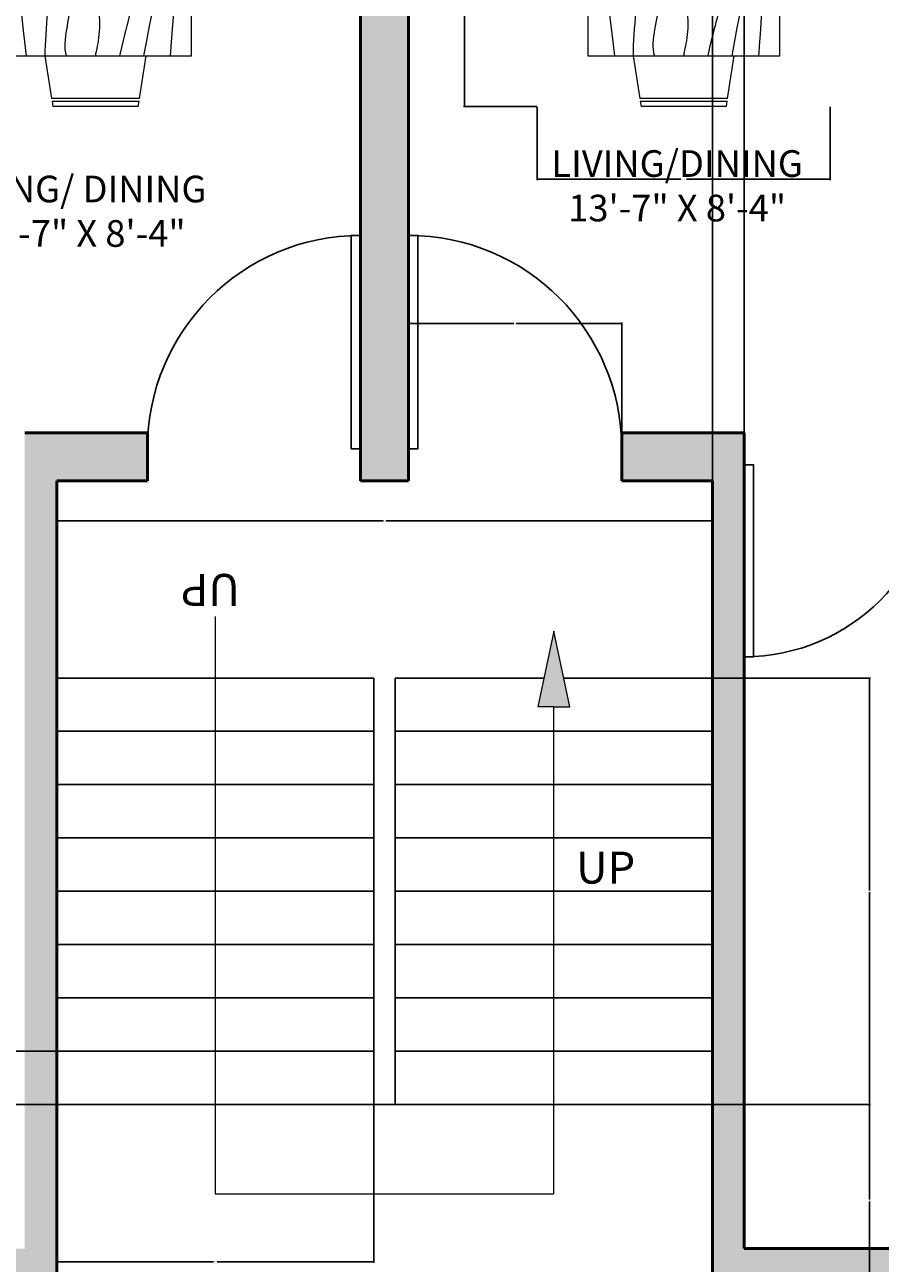
# Model space of a CAD drawing. Units: inches. Extents: x 2710 to 3197, y 524 to 1147.
# Tile 3 of 6: x 2885 to 3046, y 640 to 873. Entities that reach past the tile are written whole.
import ezdxf

# ---------------------------------------------------------------- set-up
doc = ezdxf.new("R2010")
doc.units = ezdxf.units.IN
for name, color, linetype, lineweight in [('A-ANNO-DIMS', 2, 'Continuous', 18), ('A-ANNO-SYMB', 1, 'Continuous', 18), ('A-ANNO-TEXT', 7, 'Continuous', 18), ('A-AREA-IDEN', 7, 'Continuous', 25), ('A-DOOR', 3, 'Continuous', 25), ('A-FLOR-STRS', 7, 'Continuous', 25), ('A-FURN', 8, 'Continuous', 18), ('A-WALL', 7, 'Continuous', 50), ('A-WALL-PATT', 74, 'Continuous', 13)]:
    doc.layers.add(name, color=color, linetype=linetype, lineweight=lineweight)
doc.styles.get("Standard").update_dxf_attribs({"font": 'arial.ttf'})
doc.dimstyles.get("Standard").update_dxf_attribs({"dimtxt": 0.18, "dimasz": 0.18, "dimexe": 0.18, "dimexo": 0.0625, "dimgap": 0.09, "dimtad": 0, "dimtih": 1, "dimtoh": 1, "dimdec": 4, "dimzin": 0, "dimdsep": 46, "dimtxsty": 'Standard', "dimcen": 0.09, "dimadec": 0, "dimazin": 0, "dimtfac": 1, "dimtdec": 4, "dimtofl": 0, "dimtmove": 0, "dimatfit": 3, "dimfxl": 1, "dimtolj": 1, "dimtzin": 0, "dimarcsym": 0})

# ---------------------------------------------------------------- blocks, each defined once
blk = doc.blocks.new('*U3')
for p, q in [((0, 0), (0, -6)), ((40, 0), (40, -6))]:
    blk.add_line(p, q)
blk.add_lwpolyline([(0, 0), (0, 40), (1.75, 40), (1.75, 0)], close=True)
blk.add_arc((0, 0), 40, 0, 90)
blk = doc.blocks.new('*U7')
for p, q in [((0, 0), (0, -6)), ((-40, 0), (-40, -6))]:
    blk.add_line(p, q)
blk.add_lwpolyline([(0, 0), (0, 40), (-1.75, 40), (-1.75, 0)], close=True)
blk.add_arc((0, 0), 40, 90, 180)
blk = doc.blocks.new('*U8')
for p, q in [((0, 0), (0, 6)), ((36, 0), (36, 6))]:
    blk.add_line(p, q)
blk.add_lwpolyline([(0, 0), (0, -36), (1.75, -36), (1.75, 0)], close=True)
blk.add_arc((0, 0), 36, 270, 0)
blk = doc.blocks.new('Dining Set - 36 x 72 in.')
for p, q in [((-22.2343, 26.00059), (-23.4847, 17.99762)), ((-22.2304, 26), (-5.7608, 26)), ((-22, 27.5), (-22.1562, 26.50042)), ((-5.8416, 26.5), (-22.1534, 26.5)), ((-22, 27.5), (-6, 27.5)), ((-5.8437, 26.49966), (-6, 27.5)), ((-4.5152, 17.99762), (-5.7655, 25.99926)), ((5.7657, 26.00059), (4.5153, 17.99762)), ((5.7696, 26), (22.2392, 26)), ((6, 27.5), (5.8438, 26.50042)), ((22.1584, 26.5), (5.8466, 26.5)), ((6, 27.5), (22, 27.5)), ((22.1563, 26.49966), (22, 27.5)), ((23.4848, 17.99762), (22.2345, 25.99926)), ((36, 18), (-36, 18)), ((-36, 18), (-36, -18)), ((36, -18), (36, 18)), ((-44.0006, 8.23428), (-35.9976, 9.48474)), ((44.0006, 8.23428), (35.9976, 9.48474)), ((-45.5, 8), (-44.5004, 8.15617)), ((-45.5, 8), (-45.5, -8)), ((-44.5, -8.15843), (-44.5, 8.15338)), ((-44, 8.23041), (-44, -8.23915)), ((44, 8.23041), (44, -8.23915)), ((44.5, -8.15843), (44.5, 8.15338)), ((45.5, 8), (44.5005, 8.15617)), ((45.5, 8), (45.5, -8)), ((-44.4997, -8.15631), (-45.5, -8)), ((-35.9976, -9.48476), (-43.9993, -8.2345)), ((35.9976, -9.48476), (43.9993, -8.2345)), ((44.4997, -8.15631), (45.5, -8)), ((-36, -18), (36, -18)), ((-22.2343, -26.0006), (-23.4847, -17.99762)), ((-4.5152, -17.99762), (-5.7655, -25.99928)), ((5.7657, -26.0006), (4.5153, -17.99762)), ((23.4848, -17.99762), (22.2345, -25.99928)), ((-22.2304, -26), (-5.7608, -26)), ((-22, -27.5), (-22.1562, -26.50044)), ((-5.8416, -26.5), (-22.1534, -26.5)), ((-22, -27.5), (-6, -27.5)), ((-5.8437, -26.49967), (-6, -27.5)), ((5.7696, -26), (22.2392, -26)), ((6, -27.5), (5.8438, -26.50044)), ((22.1584, -26.5), (5.8466, -26.5)), ((6, -27.5), (22, -27.5)), ((22.1563, -26.49967), (22, -27.5))]:
    blk.add_line(p, q)
for points in [[(-36, 15), (-31.1772, 14.97754), (-26.8079, 14.91406), (-22.8538, 14.81543), (-19.276, 14.6875), (-16.0362, 14.53613), (-13.0957, 14.36718), (-10.4159, 14.18652), (-7.9583, 14), (-5.6904, 13.81315), (-3.6035, 13.63021), (-1.6954, 13.45508), (0.0365, 13.29166), (1.5945, 13.14388), (2.9811, 13.01562), (4.1988, 12.9108), (5.25, 12.83333), (6.1393, 12.78613), (6.8802, 12.76823), (7.4883, 12.77767), (7.9792, 12.8125), (8.3685, 12.87077), (8.6719, 12.95052), (8.9049, 13.0498), (9.0833, 13.16666), (9.2205, 13.29899), (9.3216, 13.44401), (9.3895, 13.59879), (9.4271, 13.76041), (9.4373, 13.92594), (9.4232, 14.09245), (9.3875, 14.257), (9.3333, 14.41666), (9.2638, 14.56917), (9.1836, 14.71484), (9.0975, 14.85465), (9.0104, 14.98958), (8.9272, 15.1206), (8.8529, 15.2487), (8.7922, 15.37483), (8.75, 15.5), (8.7305, 15.62467), (8.7344, 15.74739), (8.7617, 15.86621), (8.8125, 15.97916), (8.8867, 16.08431), (8.9844, 16.17968), (9.1055, 16.26334), (9.25, 16.33333), (9.4189, 16.38802), (9.6172, 16.42708), (9.8506, 16.45052), (10.125, 16.45833), (10.4463, 16.45052), (10.8203, 16.42708), (11.2529, 16.38802), (11.75, 16.33333), (12.3184, 16.26318), (12.9694, 16.17838), (13.7151, 16.07991), (14.5677, 15.96875), (15.5395, 15.84586), (16.6426, 15.71224), (17.8893, 15.56884), (19.2917, 15.41666), (20.859, 15.25667), (22.5879, 15.08984), (24.4721, 14.91715), (26.5052, 14.73958), (28.6809, 14.5581), (30.9929, 14.3737), (33.4347, 14.18733), (36, 14)], [(-36, 10), (-28.9766, 10.14274), (-23.1725, 10.20442), (-18.4241, 10.19775), (-14.5677, 10.13541), (-11.4399, 10.03011), (-8.877, 9.89453), (-6.7154, 9.74137), (-4.7917, 9.58333), (-2.9698, 9.43082), (-1.2246, 9.28515), (0.4415, 9.14534), (2.026, 9.01041), (3.5266, 8.87939), (4.9408, 8.7513), (6.266, 8.62516), (7.5, 8.5), (8.6411, 8.37549), (9.6914, 8.2539), (10.6538, 8.13818), (11.5312, 8.03125), (12.3267, 7.93603), (13.043, 7.85547), (13.6831, 7.79248), (14.25, 7.75), (14.7471, 7.7303), (15.1797, 7.73307), (15.5537, 7.75732), (15.875, 7.80208), (16.1494, 7.86637), (16.3828, 7.94922), (16.5811, 8.04964), (16.75, 8.16666), (16.8944, 8.29915), (17.0143, 8.44531), (17.1089, 8.60319), (17.1771, 8.77083), (17.218, 8.94629), (17.2305, 9.1276), (17.2137, 9.31282), (17.1667, 9.5), (17.0895, 9.6875), (16.987, 9.875), (16.8649, 10.0625), (16.7292, 10.25), (16.5856, 10.4375), (16.4401, 10.625), (16.2985, 10.8125), (16.1667, 11), (16.05, 11.18733), (15.9518, 11.3737), (15.8752, 11.5581), (15.8229, 11.73958), (15.798, 11.91715), (15.8034, 12.08984), (15.842, 12.25667), (15.9167, 12.41666), (16.0295, 12.56836), (16.1784, 12.70833), (16.3605, 12.83268), (16.5729, 12.9375), (16.8127, 13.01888), (17.0768, 13.07291), (17.3625, 13.0957), (17.6667, 13.08333), (17.9894, 13.03312), (18.3418, 12.94726), (18.7382, 12.82918), (19.1927, 12.68229), (19.7195, 12.51001), (20.3327, 12.31575), (21.0465, 12.10294), (21.875, 11.875), (22.8357, 11.63354), (23.959, 11.37304), (25.2786, 11.08618), (26.8282, 10.76562), (28.6414, 10.40405), (30.752, 9.99414), (33.1936, 9.52856), (36, 9)], [(-36, 5.5), (-30.7157, 5.3348), (-26.069, 5.20963), (-21.9946, 5.11767), (-18.4271, 5.05208), (-15.3009, 5.00602), (-12.5508, 4.97265), (-10.1112, 4.94515), (-7.9167, 4.91666), (-5.909, 4.88167), (-4.0586, 4.83984), (-2.3429, 4.79215), (-0.7396, 4.73958), (0.7739, 4.6831), (2.22, 4.6237), (3.6213, 4.56233), (5, 4.5), (6.373, 4.43782), (7.7344, 4.3776), (9.0723, 4.32129), (10.375, 4.27083), (11.6309, 4.22819), (12.8281, 4.19531), (13.9551, 4.17415), (15, 4.16666), (15.954, 4.17448), (16.819, 4.19791), (17.6001, 4.23698), (18.3021, 4.29166), (18.9299, 4.36198), (19.4883, 4.44791), (19.9823, 4.54948), (20.4167, 4.66666), (20.7969, 4.79899), (21.1302, 4.94401), (21.4245, 5.09879), (21.6875, 5.26041), (21.9271, 5.42594), (22.1511, 5.59245), (22.3672, 5.757), (22.5834, 5.91666), (22.8065, 6.06868), (23.0404, 6.21093), (23.2879, 6.34147), (23.5521, 6.45833), (23.8358, 6.55957), (24.142, 6.64323), (24.4735, 6.70735), (24.8334, 6.75), (25.2235, 6.76969), (25.642, 6.76692), (26.0858, 6.74267), (26.5521, 6.69791), (27.0379, 6.63362), (27.5404, 6.55078), (28.0565, 6.45036), (28.5834, 6.33333), (29.1242, 6.19987), (29.7071, 6.04687), (30.3661, 5.87044), (31.1354, 5.66666), (32.0493, 5.43164), (33.142, 5.16146), (34.4475, 4.85221), (36, 4.5)], [(-36, -1), (-30.7915, -0.6591), (-26.0195, -0.38216), (-21.6519, -0.16284), (-17.6563, 0.00521), (-14.0005, 0.12833), (-10.6523, 0.21289), (-7.5796, 0.26522), (-4.75, 0.29166), (-2.134, 0.29793), (0.2878, 0.28711), (2.5317, 0.26163), (4.6146, 0.22396), (6.5529, 0.17651), (8.3633, 0.12174), (10.0623, 0.06209), (11.6667, 0), (13.1899, -0.06201), (14.6341, -0.1211), (15.9982, -0.17432), (17.2813, -0.21875), (18.4823, -0.25147), (19.6003, -0.26953), (20.6343, -0.27002), (21.5834, -0.25), (22.4481, -0.20768), (23.2357, -0.14584), (23.9549, -0.06836), (24.6146, 0.02083), (25.2235, 0.11784), (25.7904, 0.21875), (26.3241, 0.31966), (26.8334, 0.41666), (27.3265, 0.50618), (27.8099, 0.58593), (28.2894, 0.65397), (28.7709, 0.70833), (29.2601, 0.74707), (29.763, 0.76823), (30.2855, 0.76985), (30.8334, 0.75), (31.4088, 0.70784), (31.9994, 0.64713), (32.589, 0.57275), (33.1615, 0.48958), (33.7008, 0.4025), (34.1908, 0.3164), (34.6153, 0.23616), (34.9584, 0.16666), (35.2099, 0.11165), (35.3848, 0.07031), (35.504, 0.04069), (35.5886, 0.02083), (35.6594, 0.00879), (35.7377, 0.0026), (35.8442, 0.00032), (36, 0)], [(-36, -6.5), (-27.1843, -6.31267), (-20.084, -6.1263), (-14.469, -5.9419), (-10.1094, -5.76042), (-6.7752, -5.58285), (-4.2363, -5.41016), (-2.2629, -5.24333), (-0.625, -5.08334), (0.8708, -4.93099), (2.2715, -4.78646), (3.5872, -4.64974), (4.8281, -4.52084), (6.0046, -4.39974), (7.127, -4.28646), (8.2053, -4.18099), (9.25, -4.08334), (10.2705, -3.99382), (11.2734, -3.91407), (12.2647, -3.84603), (13.25, -3.79167), (14.2354, -3.75293), (15.2266, -3.73177), (16.2295, -3.73015), (17.25, -3.75), (18.2912, -3.79248), (19.3451, -3.85547), (20.4009, -3.93604), (21.4479, -4.03125), (22.4754, -4.13819), (23.4727, -4.25391), (24.4289, -4.37549), (25.3334, -4.5), (26.1785, -4.62492), (26.9694, -4.74935), (27.7145, -4.87281), (28.4219, -4.99479), (29.1, -5.11483), (29.7572, -5.23242), (30.4016, -5.34709), (31.0417, -5.45834), (31.6837, -5.56437), (32.3262, -5.65821), (32.9658, -5.73153), (33.599, -5.77604), (34.2224, -5.78345), (34.8327, -5.74545), (35.4264, -5.65373), (36, -5.5)], [(-36, -10), (-26.4022, -9.81299), (-18.4675, -9.62891), (-11.9839, -9.45069), (-6.7396, -9.28125), (-2.5226, -9.12354), (0.8789, -8.98047), (3.6769, -8.85498), (6.0833, -8.75), (8.2767, -8.66765), (10.3021, -8.60677), (12.1712, -8.56543), (13.8958, -8.54167), (15.4876, -8.53353), (16.9583, -8.53907), (18.3197, -8.55632), (19.5834, -8.58334), (20.7616, -8.61841), (21.8685, -8.66081), (22.9188, -8.71004), (23.9271, -8.76563), (24.9081, -8.82707), (25.8763, -8.89388), (26.8465, -8.96558), (27.8334, -9.04167), (28.8474, -9.12118), (29.8828, -9.20117), (30.93, -9.27824), (31.9792, -9.34896), (33.0205, -9.40991), (34.0443, -9.45768), (35.0407, -9.48885), (36, -9.5)], [(-36, -14.5), (-30.0881, -14.33513), (-25.0332, -14.21224), (-20.7312, -14.12647), (-17.0781, -14.07292), (-13.97, -14.04671), (-11.3027, -14.04297), (-8.9724, -14.05681), (-6.875, -14.08334), (-4.9224, -14.11833), (-3.0905, -14.16016), (-1.3709, -14.20785), (0.2448, -14.26042), (1.7647, -14.3169), (3.1973, -14.3763), (4.5507, -14.43767), (5.8333, -14.5), (7.0554, -14.5621), (8.235, -14.62175), (9.3922, -14.67652), (10.5469, -14.72396), (11.7192, -14.76164), (12.929, -14.78711), (14.1965, -14.79794), (15.5417, -14.79167), (16.9933, -14.76424), (18.6152, -14.70508), (20.4804, -14.60197), (22.6615, -14.44271), (25.2312, -14.21509), (28.2624, -13.9069), (31.8277, -13.50594), (36, -13)]]:
    blk.add_lwpolyline(points)
blk = doc.blocks.new('*D26')
at = {"layer": 'A-ANNO-DIMS', "color": 0, "lineweight": -2, "transparency": 16777216}
for p, q in [((2981.42, 948.17), (2967.65, 948.17)), ((2967.83, 947.99), (2967.83, 902.86)), ((2967.83, 857.35), (2967.83, 902.49)), ((2981.42, 857.17), (2967.65, 857.17))]:
    blk.add_line(p, q, dxfattribs=at)
at = {"layer": 'A-ANNO-DIMS', "color": 0, "transparency": 16777216}
for points in [[(2967.8, 947.99), (2967.86, 947.99), (2967.83, 948.17)], [(2967.8, 857.35), (2967.86, 857.35), (2967.83, 857.17)]]:
    blk.add_solid(points, dxfattribs=at)
at = {"layer": 'Defpoints', "color": 0, "transparency": 16777216}
for p in [(2981.48, 948.17), (2967.83, 857.17), (2981.48, 857.17)]:
    blk.add_point(p, dxfattribs=at)
at = {"layer": 'A-ANNO-DIMS', "color": 0, "transparency": 16777216, "insert": (2967.83, 902.67), "char_height": 0.18, "attachment_point": 5}
blk.add_mtext('\\A1;DINING SET 91 TYP.', dxfattribs=at)
blk = doc.blocks.new('*D27')
at = {"layer": 'A-ANNO-DIMS', "color": 0, "lineweight": -2, "transparency": 16777216}
for p, q in [((2981.48, 857.11), (2981.48, 843.34)), ((3036.48, 857.11), (3036.48, 843.34)), ((2981.66, 843.52), (3008.45, 843.52)), ((3036.3, 843.52), (3009.51, 843.52))]:
    blk.add_line(p, q, dxfattribs=at)
at = {"layer": 'A-ANNO-DIMS', "color": 0, "transparency": 16777216}
for points in [[(2981.66, 843.55), (2981.66, 843.49), (2981.48, 843.52)], [(3036.3, 843.55), (3036.3, 843.49), (3036.48, 843.52)]]:
    blk.add_solid(points, dxfattribs=at)
at = {"layer": 'Defpoints', "color": 0, "transparency": 16777216}
for p in [(2981.48, 857.17), (3036.48, 857.17), (3036.48, 843.52)]:
    blk.add_point(p, dxfattribs=at)
at = {"layer": 'A-ANNO-DIMS', "color": 0, "transparency": 16777216, "insert": (3008.98, 843.52), "char_height": 0.18, "attachment_point": 5}
blk.add_mtext('\\A1;55 TYP.', dxfattribs=at)
blk = doc.blocks.new('*D70')
at = {"layer": 'A-ANNO-DIMS', "color": 0, "lineweight": -2, "transparency": 16777216}
for p, q in [((2891.35, 750.06), (2891.35, 779.68)), ((2891.53, 779.5), (2952.57, 779.5)), ((3014.17, 779.5), (2953.13, 779.5)), ((3014.35, 750.06), (3014.35, 779.68))]:
    blk.add_line(p, q, dxfattribs=at)
at = {"layer": 'A-ANNO-DIMS', "color": 0, "transparency": 16777216}
for points in [[(2891.53, 779.53), (2891.53, 779.47), (2891.35, 779.5)], [(3014.17, 779.53), (3014.17, 779.47), (3014.35, 779.5)]]:
    blk.add_solid(points, dxfattribs=at)
at = {"layer": 'Defpoints', "color": 0, "transparency": 16777216}
for p in [(3014.35, 779.5), (2891.35, 750), (3014.35, 750)]:
    blk.add_point(p, dxfattribs=at)
at = {"layer": 'A-ANNO-DIMS', "color": 0, "transparency": 16777216, "insert": (2952.85, 779.5), "char_height": 0.18, "attachment_point": 5}
blk.add_mtext('\\A1;123', dxfattribs=at)
blk = doc.blocks.new('*D71')
at = {"layer": 'A-ANNO-DIMS', "color": 0, "lineweight": -2, "transparency": 16777216}
for p, q in [((3014.41, 670), (3044.03, 670)), ((3043.85, 669.82), (3043.85, 652.18)), ((3043.85, 634.18), (3043.85, 651.82)), ((3014.41, 634), (3044.03, 634))]:
    blk.add_line(p, q, dxfattribs=at)
at = {"layer": 'A-ANNO-DIMS', "color": 0, "transparency": 16777216}
for points in [[(3043.82, 669.82), (3043.88, 669.82), (3043.85, 670)], [(3043.82, 634.18), (3043.88, 634.18), (3043.85, 634)]]:
    blk.add_solid(points, dxfattribs=at)
at = {"layer": 'Defpoints', "color": 0, "transparency": 16777216}
for p in [(3014.35, 670), (3014.35, 634), (3043.85, 634)]:
    blk.add_point(p, dxfattribs=at)
at = {"layer": 'A-ANNO-DIMS', "color": 0, "transparency": 16777216, "insert": (3043.85, 652), "char_height": 0.18, "attachment_point": 5}
blk.add_mtext('\\A1;36', dxfattribs=at)
blk = doc.blocks.new('*D72')
at = {"layer": 'A-ANNO-DIMS', "color": 0, "lineweight": -2, "transparency": 16777216}
for p, q in [((3014.41, 750), (3044.03, 750)), ((3043.85, 749.82), (3043.85, 710.18)), ((3043.85, 670.18), (3043.85, 709.82)), ((3014.41, 670), (3044.03, 670))]:
    blk.add_line(p, q, dxfattribs=at)
at = {"layer": 'A-ANNO-DIMS', "color": 0, "transparency": 16777216}
for points in [[(3043.82, 749.82), (3043.88, 749.82), (3043.85, 750)], [(3043.82, 670.18), (3043.88, 670.18), (3043.85, 670)]]:
    blk.add_solid(points, dxfattribs=at)
at = {"layer": 'Defpoints', "color": 0, "transparency": 16777216}
for p in [(3014.35, 750), (3014.35, 670), (3043.85, 670)]:
    blk.add_point(p, dxfattribs=at)
at = {"layer": 'A-ANNO-DIMS', "color": 0, "transparency": 16777216, "insert": (3043.85, 710), "char_height": 0.18, "attachment_point": 5}
blk.add_mtext('\\A1;80', dxfattribs=at)
blk = doc.blocks.new('*D73')
at = {"layer": 'A-ANNO-DIMS', "color": 0, "lineweight": -2, "transparency": 16777216}
for p, q in [((2957.35, 787.06), (2957.35, 816.68)), ((2957.53, 816.5), (2977.13, 816.5)), ((2997.17, 816.5), (2977.57, 816.5)), ((2997.35, 787.06), (2997.35, 816.68))]:
    blk.add_line(p, q, dxfattribs=at)
at = {"layer": 'A-ANNO-DIMS', "color": 0, "transparency": 16777216}
for points in [[(2957.53, 816.53), (2957.53, 816.47), (2957.35, 816.5)], [(2997.17, 816.53), (2997.17, 816.47), (2997.35, 816.5)]]:
    blk.add_solid(points, dxfattribs=at)
at = {"layer": 'Defpoints', "color": 0, "transparency": 16777216}
for p in [(2997.35, 816.5), (2957.35, 787), (2997.35, 787)]:
    blk.add_point(p, dxfattribs=at)
at = {"layer": 'A-ANNO-DIMS', "color": 0, "transparency": 16777216, "insert": (2977.35, 816.5), "char_height": 0.18, "attachment_point": 5}
blk.add_mtext('\\A1;40', dxfattribs=at)
blk = doc.blocks.new('*D79')
at = {"layer": 'A-ANNO-DIMS', "color": 0, "lineweight": -2, "transparency": 16777216}
for p, q in [((3014.35, 787.06), (3014.35, 1146.99)), ((3014.53, 1146.81), (3017.2, 1146.81)), ((3020.17, 1146.81), (3017.5, 1146.81)), ((3020.35, 796.06), (3020.35, 1146.99))]:
    blk.add_line(p, q, dxfattribs=at)
at = {"layer": 'A-ANNO-DIMS', "color": 0, "transparency": 16777216}
for points in [[(3014.53, 1146.84), (3014.53, 1146.78), (3014.35, 1146.81)], [(3020.17, 1146.84), (3020.17, 1146.78), (3020.35, 1146.81)]]:
    blk.add_solid(points, dxfattribs=at)
at = {"layer": 'Defpoints', "color": 0, "transparency": 16777216}
for p in [(3020.35, 1146.81), (3020.35, 796), (3014.35, 787)]:
    blk.add_point(p, dxfattribs=at)
at = {"layer": 'A-ANNO-DIMS', "color": 0, "transparency": 16777216, "insert": (3017.35, 1146.81), "char_height": 0.18, "attachment_point": 5}
blk.add_mtext('\\A1;6', dxfattribs=at)
blk = doc.blocks.new('*D80')
at = {"layer": 'A-ANNO-DIMS', "color": 0, "lineweight": -2, "transparency": 16777216}
for p, q in [((2891.29, 680), (2861.67, 680)), ((2861.85, 679.82), (2861.85, 675.18)), ((2861.85, 670.18), (2861.85, 674.82)), ((2891.29, 670), (2861.67, 670))]:
    blk.add_line(p, q, dxfattribs=at)
at = {"layer": 'A-ANNO-DIMS', "color": 0, "transparency": 16777216}
for points in [[(2861.82, 679.82), (2861.88, 679.82), (2861.85, 680)], [(2861.82, 670.18), (2861.88, 670.18), (2861.85, 670)]]:
    blk.add_solid(points, dxfattribs=at)
at = {"layer": 'Defpoints', "color": 0, "transparency": 16777216}
for p in [(2861.85, 680), (2891.35, 680), (2891.35, 670)]:
    blk.add_point(p, dxfattribs=at)
at = {"layer": 'A-ANNO-DIMS', "color": 0, "transparency": 16777216, "insert": (2861.85, 675), "char_height": 0.18, "attachment_point": 5}
blk.add_mtext('\\A1;10', dxfattribs=at)
blk = doc.blocks.new('*D81')
at = {"layer": 'A-ANNO-DIMS', "color": 0, "lineweight": -2, "transparency": 16777216}
for p, q in [((2891.35, 669.94), (2891.35, 640.32)), ((2950.85, 669.94), (2950.85, 640.32)), ((2891.53, 640.5), (2920.77, 640.5)), ((2950.67, 640.5), (2921.42, 640.5))]:
    blk.add_line(p, q, dxfattribs=at)
at = {"layer": 'A-ANNO-DIMS', "color": 0, "transparency": 16777216}
for points in [[(2891.53, 640.53), (2891.53, 640.47), (2891.35, 640.5)], [(2950.67, 640.53), (2950.67, 640.47), (2950.85, 640.5)]]:
    blk.add_solid(points, dxfattribs=at)
at = {"layer": 'Defpoints', "color": 0, "transparency": 16777216}
for p in [(2891.35, 670), (2950.85, 670), (2891.35, 640.5)]:
    blk.add_point(p, dxfattribs=at)
at = {"layer": 'A-ANNO-DIMS', "color": 0, "transparency": 16777216, "insert": (2921.1, 640.5), "char_height": 0.18, "attachment_point": 5}
blk.add_mtext('\\A1;59.5', dxfattribs=at)

msp = doc.modelspace()

# ---------------------------------------------------------------- hatches: boundary and pattern name
at = {"layer": 'A-ANNO-SYMB'}
h = msp.add_hatch(color=256, dxfattribs=at)
h.dxf.hatch_style = 1
h.paths.add_polyline_path([(2984.5984, 758.7655), (2981.5984, 744.5654), (2984.5984, 744.5654), (2987.5984, 744.5654)])
at = {"layer": 'A-WALL-PATT'}
h = msp.add_hatch(color=256, dxfattribs=at)
h.dxf.hatch_style = 1
h.paths.add_polyline_path([(2898.3484, 1096.0017), (2898.3484, 967.0017), (2948.3484, 967.0017), (2948.3484, 787.0017), (2957.3484, 787.0017), (2957.3484, 793.0017), (2957.3484, 833.0017), (2957.3484, 967.0017), (3007.3484, 967.0017), (3007.3484, 973.0017), (3007.3484, 1009.0017), (3007.3484, 1096.0017), (3149.3484, 1096.0017), (3149.3484, 1084.4601), (3158.3484, 1084.4601), (3158.3484, 1105.0017), (2991.781, 1105.0017), (2991.781, 1096.0017), (2998.3484, 1096.0017), (2998.3484, 976.0017), (2957.3484, 976.0017), (2957.3484, 1003.0017), (2966.3484, 1003.0017), (2966.3484, 1012.0017), (2957.3484, 1012.0017), (2957.3484, 1096.0017), (2963.4487, 1096.0017), (2963.4487, 1105.0017), (2940.703, 1105.0017), (2940.703, 1096.0017), (2948.3484, 1096.0017), (2948.3484, 1012.0017), (2939.3484, 1012.0017), (2939.3484, 1003.0017), (2948.3484, 1003.0017), (2948.3484, 976.0017), (2907.3484, 976.0017), (2907.3484, 1096.0017), (2916.9598, 1096.0017), (2916.9598, 1105.0017), (2857.03, 1105.0017), (2857.03, 1096.0017)])
h.paths.add_polyline_path([(2789.8274, 1096.0017), (2789.8274, 1105.0017), (2747.3484, 1105.0017), (2747.3484, 943.327), (2756.3484, 943.327), (2756.3484, 967.0017), (2828.3484, 967.0017), (2828.3484, 909.0017), (2837.3484, 909.0017), (2837.3484, 967.0017), (2862.3484, 967.0017), (2862.3484, 973.0017), (2862.3484, 976.0017), (2756.3484, 976.0017), (2756.3484, 1096.0017)])
h.paths.add_polyline_path([(2828.3484, 868.0017), (2828.3484, 830.0017), (2837.3484, 830.0017), (2837.3484, 877.0017), (2756.3484, 877.0017), (2756.3484, 904.8338), (2747.3484, 904.8338), (2747.3484, 858.8554), (2756.3484, 858.8554), (2756.3484, 868.0017)])
h.paths.add_polyline_path([(2747.3484, 742.5572), (2756.3484, 742.5572), (2756.3484, 787.0017), (2849.3484, 787.0017), (2849.3484, 796.0017), (2837.3484, 796.0017), (2837.3484, 802.0017), (2831.3484, 802.0017), (2828.3484, 802.0017), (2828.3484, 796.0017), (2756.3484, 796.0017), (2756.3484, 819.3052), (2747.3484, 819.3052)])
h.paths.add_polyline_path([(2756.3484, 643.0017), (2756.3484, 672.4477), (2747.3484, 672.4477), (2747.3484, 565.0017), (2825.5051, 565.0017), (2825.5051, 574.0017), (2756.3484, 574.0017), (2756.3484, 634.0017), (2891.3484, 634.0017), (2891.3484, 787.0017), (2908.3484, 787.0017), (2908.3484, 793.0017), (2908.3484, 796.0017), (2891.3484, 796.0017), (2885.3484, 796.0017), (2885.3484, 790.0017), (2885.3484, 754.0017), (2885.3484, 643.0017)])
h.paths.add_polyline_path([(2924.8484, 565.0017), (2924.8484, 571.0017), (2924.8484, 574.0017), (2872.3715, 574.0017), (2872.3715, 565.0017)])
h.paths.add_polyline_path([(2984.8484, 574.0017), (2984.8484, 571.0017), (2984.8484, 565.0017), (3050.793, 565.0017), (3050.793, 574.0017)])
h.paths.add_polyline_path([(3158.3484, 565.0017), (3158.3484, 685.5326), (3149.3484, 685.5326), (3149.3484, 675.4542), (3149.3484, 643.0017), (3020.3484, 643.0017), (3020.3484, 796.0017), (3014.3484, 796.0017), (2997.3484, 796.0017), (2997.3484, 787.0017), (3014.3484, 787.0017), (3014.3484, 634.0017), (3149.3484, 634.0017), (3149.3484, 574.0017), (3104.3903, 574.0017), (3104.3903, 565.0017)])
h.paths.add_polyline_path([(3149.3484, 787.0017), (3149.3484, 746.9465), (3158.3484, 746.9465), (3158.3484, 820.3805), (3149.3484, 820.3805), (3149.3484, 796.0017), (3077.3484, 796.0017), (3077.3484, 802.0017), (3074.3484, 802.0017), (3068.3484, 802.0017), (3068.3484, 796.0017), (3056.3484, 796.0017), (3056.3484, 790.0017), (3056.3484, 787.0017)])
h.paths.add_polyline_path([(3158.3484, 905.224), (3149.3484, 905.224), (3149.3484, 877.0017), (3068.3484, 877.0017), (3068.3484, 838.0017), (3074.3484, 838.0017), (3077.3484, 838.0017), (3077.3484, 868.0017), (3149.3484, 868.0017), (3149.3484, 852.3022), (3158.3484, 852.3022)], flags=17)
h.paths.add_polyline_path([(3099.2867, 814.3126), (3142.0289, 814.3126), (3142.0289, 832.97), (3099.2867, 832.97)], flags=25)
h.paths.add_polyline_path([(2981.8144, 832.8032), (3033.605, 832.8032), (3033.605, 851.4605), (2981.8144, 851.4605)], flags=25)

# ---------------------------------------------------------------- linework, layer by layer
at = {"layer": 'A-ANNO-SYMB'}
for p, q in [((2921.0984, 761.5045), (2921.0984, 653.2423)), ((2984.5984, 758.7655), (2981.5984, 744.5654)), ((2987.5984, 744.5654), (2984.5984, 758.7655)), ((2984.5984, 744.5654), (2981.5984, 744.5654)), ((2984.5984, 653.2423), (2984.5984, 744.5654)), ((2984.5984, 744.5654), (2987.5984, 744.5654)), ((2921.0984, 653.2423), (2984.5984, 653.2423))]:
    msp.add_line(p, q, dxfattribs=at)
at = {"layer": 'A-FLOR-STRS'}
for p, q in [((2950.8484, 750.0017), (2891.3484, 750.0017)), ((2950.8484, 670.0017), (2950.8484, 750.0017)), ((2954.8484, 670.0017), (2954.8484, 750.0017)), ((2982.7469, 750.0017), (2954.8484, 750.0017)), ((3014.3484, 750.0017), (2986.4499, 750.0017)), ((2950.8484, 740.0017), (2891.3484, 740.0017)), ((3014.3484, 740.0017), (2954.8484, 740.0017)), ((2950.8484, 730.0017), (2891.3484, 730.0017)), ((3014.3484, 730.0017), (2954.8484, 730.0017)), ((2950.8484, 720.0017), (2891.3484, 720.0017)), ((3014.3484, 720.0017), (2954.8484, 720.0017)), ((2950.8484, 710.0017), (2891.3484, 710.0017)), ((3014.3484, 710.0017), (2954.8484, 710.0017)), ((2950.8484, 700.0017), (2891.3484, 700.0017)), ((3014.3484, 700.0017), (2954.8484, 700.0017)), ((2950.8484, 690.0017), (2891.3484, 690.0017)), ((3014.3484, 690.0017), (2954.8484, 690.0017)), ((2950.8484, 680.0017), (2891.3484, 680.0017)), ((3014.3484, 680.0017), (2954.8484, 680.0017)), ((3014.3484, 670.0017), (2891.3484, 670.0017))]:
    msp.add_line(p, q, dxfattribs=at)
at = {"layer": 'A-WALL'}
for p, q in [((2948.3484, 967.0017), (2948.3484, 787.0017)), ((2957.3484, 787.0017), (2957.3484, 967.0017)), ((2891.3484, 796.0017), (2885.3484, 796.0017)), ((2891.3484, 796.0017), (2908.3484, 796.0017)), ((2908.3484, 796.0017), (2908.3484, 787.0017)), ((3014.3484, 796.0017), (2997.3484, 796.0017)), ((2997.3484, 796.0017), (2997.3484, 787.0017)), ((3020.3484, 796.0017), (3014.3484, 796.0017)), ((3020.3484, 643.0017), (3020.3484, 796.0017)), ((2891.3484, 787.0017), (2891.3484, 634.0017)), ((2908.3484, 787.0017), (2891.3484, 787.0017)), ((2957.3484, 787.0017), (2948.3484, 787.0017)), ((2997.3484, 787.0017), (3014.3484, 787.0017)), ((3014.3484, 634.0017), (3014.3484, 787.0017)), ((3149.3484, 643.0017), (3020.3484, 643.0017))]:
    msp.add_line(p, q, dxfattribs=at)

# ---------------------------------------------------------------- block references
at = {"layer": 'A-DOOR'}
for name, p in [('*U7', (2948.3484, 793.0017)), ('*U3', (2957.3484, 793.0017)), ('*U8', (3020.3484, 790.0017))]:
    msp.add_blockref(name, p, dxfattribs=at)
at = {"layer": 'A-FURN', "rotation": 270}
for p in [(2898.63, 902.6723), (3008.9802, 902.6723)]:
    msp.add_blockref('Dining Set - 36 x 72 in.', p, dxfattribs=at)

# ---------------------------------------------------------------- texts
at = {"layer": 'A-ANNO-TEXT', "insert": (2925.7095, 763.5088), "char_height": 6, "attachment_point": 1, "rotation": 180}
msp.add_mtext_dynamic_manual_height_columns('UP', width=10.461401, gutter_width=12.5, heights=[0], dxfattribs=at)
at = {"layer": 'A-ANNO-TEXT', "insert": (2988.787, 717.4471), "char_height": 6, "attachment_point": 1}
msp.add_mtext_dynamic_manual_height_columns('UP', width=10.461401, gutter_width=12.5, heights=[0], dxfattribs=at)
at = {"layer": 'A-AREA-IDEN', "char_height": 5, "attachment_point": 1}
for s, insert in [('\\pxqc;LIVING/DINING\\P13\'-7" X 8\'-4"', (2978.9193, 848.9725)), ('\\pxqc;LIVING/ DINING\\P13\'-7" X 8\'-4"', (2866.2582, 844.202))]:
    msp.add_mtext_dynamic_manual_height_columns(s, width=57.655828, gutter_width=12.5, heights=[0], dxfattribs=dict(at, insert=insert))

# ---------------------------------------------------------------- dimensions: what is measured, and where the dimension line sits
at = {"layer": 'A-ANNO-DIMS'}
for base, p1, p2, picture, middle in [((3020.3484, 1146.8081), (3014.3484, 787.0017), (3020.3484, 796.0017), '*D79', (3017.3484, 1146.8081)), ((3014.3484, 779.5017), (2891.3484, 750.0017), (3014.3484, 750.0017), '*D70', (2952.8484, 779.5017))]:
    dim = msp.add_linear_dim(base=base, p1=p1, p2=p2, dimstyle='Standard', override={"dimdec": 0, "dimlfac": 1, "dimrnd": 0, "dimzin": 0, "dimdsep": 46, "dimlunit": 2}, dxfattribs=at)
    dim.commit()
    dim.dimension.update_dxf_attribs({"geometry": picture, "text_midpoint": middle})
dim = msp.add_linear_dim(base=(2967.8302, 857.1723), p1=(2981.4802, 948.1723), p2=(2981.4802, 857.1723), angle=270, text='DINING SET <> TYP.', dimstyle='Standard', override={"dimdec": 0, "dimlfac": 1, "dimrnd": 0, "dimzin": 0, "dimdsep": 46, "dimlunit": 2}, dxfattribs=at)
dim.commit()
dim.dimension.update_dxf_attribs({"geometry": '*D26', "text_midpoint": (2967.8302, 902.6723)})
dim = msp.add_linear_dim(base=(3036.4802, 843.5223), p1=(2981.4802, 857.1723), p2=(3036.4802, 857.1723), text='<> TYP.', dimstyle='Standard', override={"dimdec": 0, "dimlfac": 1, "dimrnd": 0, "dimzin": 0, "dimdsep": 46, "dimlunit": 2}, dxfattribs=at)
dim.commit()
dim.dimension.update_dxf_attribs({"geometry": '*D27', "text_midpoint": (3008.9802, 843.5223)})
for base, p1, p2, angle, override, picture, middle in [((2997.3484, 816.5017), (2957.3484, 787.0017), (2997.3484, 787.0017), 0, {"dimdec": 0, "dimlfac": 1, "dimrnd": 0, "dimzin": 0, "dimdsep": 46, "dimlunit": 2}, '*D73', (2977.3484, 816.5017)), ((3043.8484, 670.0017), (3014.3484, 750.0017), (3014.3484, 670.0017), 270, {"dimdec": 0, "dimlfac": 1, "dimrnd": 0, "dimzin": 0, "dimdsep": 46, "dimlunit": 2}, '*D72', (3043.8484, 710.0017)), ((2861.8484, 680.0017), (2891.3484, 670.0017), (2891.3484, 680.0017), 90, {"dimdec": 0, "dimlfac": 1, "dimrnd": 0, "dimzin": 0, "dimdsep": 46, "dimlunit": 2}, '*D80', (2861.8484, 675.0017)), ((2891.3484, 640.5017), (2950.8484, 670.0017), (2891.3484, 670.0017), 180, {"dimdec": 1, "dimlfac": 1, "dimrnd": 0, "dimzin": 0, "dimdsep": 46, "dimlunit": 2}, '*D81', (2921.0984, 640.5017)), ((3043.8484, 634.0017), (3014.3484, 670.0017), (3014.3484, 634.0017), 270, {"dimdec": 0, "dimlfac": 1, "dimrnd": 0, "dimzin": 0, "dimdsep": 46, "dimlunit": 2}, '*D71', (3043.8484, 652.0017))]:
    dim = msp.add_linear_dim(base=base, p1=p1, p2=p2, angle=angle, dimstyle='Standard', override=override, dxfattribs=at)
    dim.commit()
    dim.dimension.update_dxf_attribs({"geometry": picture, "text_midpoint": middle})

doc.saveas('drawing.dxf')
